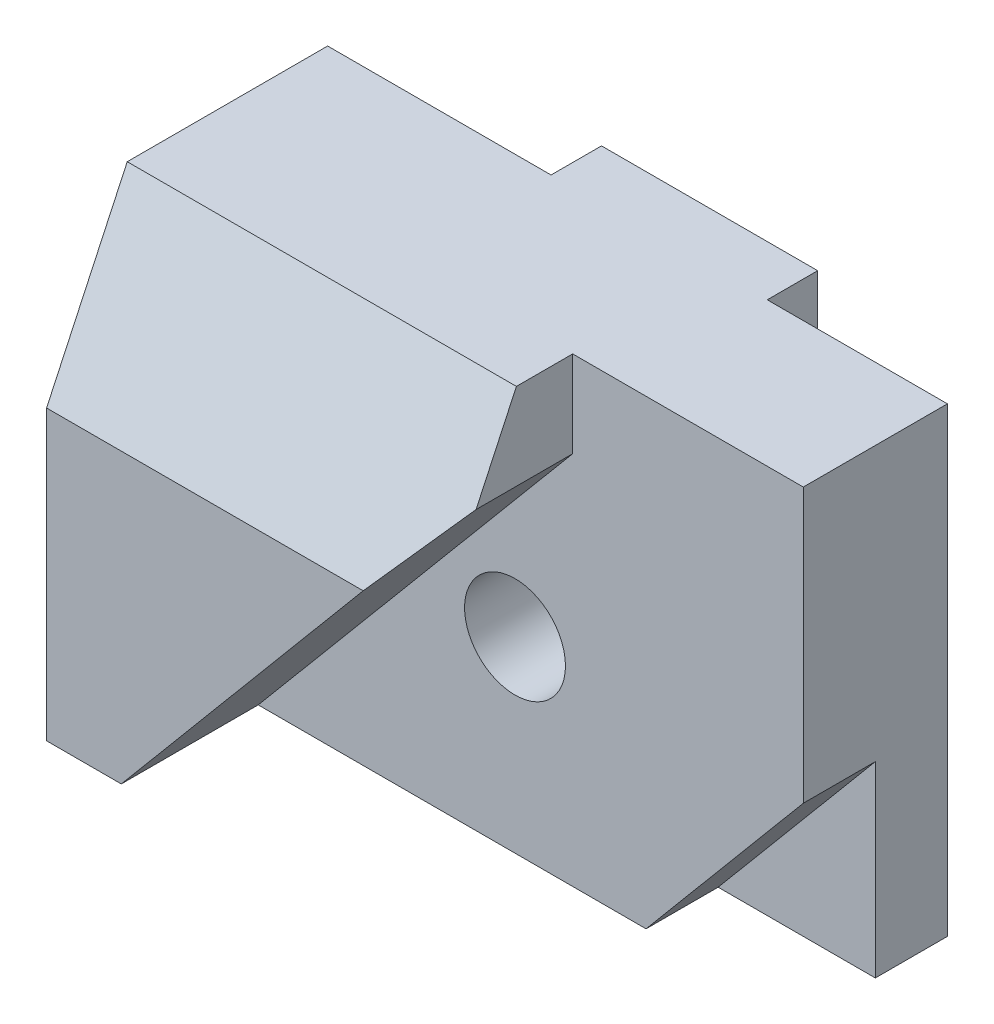
ISO-10303-21;
HEADER;
FILE_DESCRIPTION(('STEP AP214'),'2;1');
FILE_NAME('part.step','',(''),(''),'','','');
FILE_SCHEMA(('AUTOMOTIVE_DESIGN { 1 0 10303 214 1 1 1 1 }'));
ENDSEC;
DATA;
#1=APPLICATION_CONTEXT('core data for automotive mechanical design processes');
#2=APPLICATION_PROTOCOL_DEFINITION('international standard','automotive_design',2000,#1);
#3=PRODUCT_CONTEXT('',#1,'mechanical');
#4=PRODUCT('Part','Part','',(#3));
#5=PRODUCT_RELATED_PRODUCT_CATEGORY('part','',(#4));
#6=PRODUCT_DEFINITION_FORMATION('','',#4);
#7=PRODUCT_DEFINITION_CONTEXT('part definition',#1,'design');
#8=PRODUCT_DEFINITION('design','',#6,#7);
#9=PRODUCT_DEFINITION_SHAPE('','',#8);
#10=(LENGTH_UNIT() NAMED_UNIT(*) SI_UNIT(.MILLI.,.METRE.));
#11=(NAMED_UNIT(*) PLANE_ANGLE_UNIT() SI_UNIT($,.RADIAN.));
#12=(NAMED_UNIT(*) SI_UNIT($,.STERADIAN.) SOLID_ANGLE_UNIT());
#13=UNCERTAINTY_MEASURE_WITH_UNIT(LENGTH_MEASURE(1.E-05),#10,'distance_accuracy_value','');
#14=(GEOMETRIC_REPRESENTATION_CONTEXT(3) GLOBAL_UNCERTAINTY_ASSIGNED_CONTEXT((#13)) GLOBAL_UNIT_ASSIGNED_CONTEXT((#10,
#11,#12)) REPRESENTATION_CONTEXT('',''));
#15=CARTESIAN_POINT('',(0.,0.,0.));
#16=DIRECTION('',(0.,0.,1.));
#17=DIRECTION('',(1.,0.,0.));
#18=AXIS2_PLACEMENT_3D('',#15,#16,#17);
#19=CARTESIAN_POINT('',(0.,0.,0.));
#20=DIRECTION('',(0.,0.,-1.));
#21=DIRECTION('',(-1.,0.,0.));
#22=AXIS2_PLACEMENT_3D('',#19,#20,#21);
#23=PLANE('',#22);
#24=DIRECTION('',(-1.,0.,0.));
#25=VECTOR('',#24,1.);
#26=CARTESIAN_POINT('',(0.,64.,0.));
#27=LINE('',#26,#25);
#28=CARTESIAN_POINT('',(31.,64.,0.));
#29=VERTEX_POINT('',#28);
#30=CARTESIAN_POINT('',(0.,64.,0.));
#31=VERTEX_POINT('',#30);
#32=EDGE_CURVE('E178',#29,#31,#27,.T.);
#33=ORIENTED_EDGE('',*,*,#32,.F.);
#34=DIRECTION('',(0.,-1.,0.));
#35=VECTOR('',#34,1.);
#36=CARTESIAN_POINT('',(31.,64.,0.));
#37=LINE('',#36,#35);
#38=CARTESIAN_POINT('',(31.,0.,0.));
#39=VERTEX_POINT('',#38);
#40=EDGE_CURVE('E166',#29,#39,#37,.T.);
#41=ORIENTED_EDGE('',*,*,#40,.T.);
#42=DIRECTION('',(1.,0.,0.));
#43=VECTOR('',#42,1.);
#44=CARTESIAN_POINT('',(86.,0.,0.));
#45=LINE('',#44,#43);
#46=CARTESIAN_POINT('',(0.,0.,0.));
#47=VERTEX_POINT('',#46);
#48=EDGE_CURVE('E203',#47,#39,#45,.T.);
#49=ORIENTED_EDGE('',*,*,#48,.F.);
#50=DIRECTION('',(0.,-1.,0.));
#51=VECTOR('',#50,1.);
#52=CARTESIAN_POINT('',(0.,0.,0.));
#53=LINE('',#52,#51);
#54=EDGE_CURVE('E179',#31,#47,#53,.T.);
#55=ORIENTED_EDGE('',*,*,#54,.F.);
#56=EDGE_LOOP('',(#33,#41,#49,#55));
#57=FACE_BOUND('',#56,.T.);
#58=ADVANCED_FACE('F50',(#57),#23,.T.);
#59=CARTESIAN_POINT('',(0.,0.,20.));
#60=DIRECTION('',(0.,0.,1.));
#61=DIRECTION('',(1.,0.,0.));
#62=AXIS2_PLACEMENT_3D('',#59,#60,#61);
#63=PLANE('',#62);
#64=DIRECTION('',(-0.64278760968654,-0.766044443118977,0.));
#65=VECTOR('',#64,1.);
#66=CARTESIAN_POINT('',(86.,26.,20.));
#67=LINE('',#66,#65);
#68=CARTESIAN_POINT('',(86.,26.,20.));
#69=VERTEX_POINT('',#68);
#70=CARTESIAN_POINT('',(64.1834095893907,0.,20.));
#71=VERTEX_POINT('',#70);
#72=EDGE_CURVE('E248',#69,#71,#67,.T.);
#73=ORIENTED_EDGE('',*,*,#72,.F.);
#74=DIRECTION('',(0.,1.,0.));
#75=VECTOR('',#74,1.);
#76=CARTESIAN_POINT('',(86.,0.,20.));
#77=LINE('',#76,#75);
#78=CARTESIAN_POINT('',(86.,64.,20.));
#79=VERTEX_POINT('',#78);
#80=EDGE_CURVE('E204',#69,#79,#77,.T.);
#81=ORIENTED_EDGE('',*,*,#80,.T.);
#82=DIRECTION('',(-1.,0.,0.));
#83=VECTOR('',#82,1.);
#84=CARTESIAN_POINT('',(86.,64.,20.));
#85=LINE('',#84,#83);
#86=CARTESIAN_POINT('',(54.,64.,20.));
#87=VERTEX_POINT('',#86);
#88=EDGE_CURVE('E209',#79,#87,#85,.T.);
#89=ORIENTED_EDGE('',*,*,#88,.T.);
#90=DIRECTION('',(0.,-1.,0.));
#91=VECTOR('',#90,1.);
#92=CARTESIAN_POINT('',(54.,0.,20.));
#93=LINE('',#92,#91);
#94=CARTESIAN_POINT('',(54.,52.,20.));
#95=VERTEX_POINT('',#94);
#96=EDGE_CURVE('E219',#87,#95,#93,.T.);
#97=ORIENTED_EDGE('',*,*,#96,.T.);
#98=DIRECTION('',(-0.64278760968654,-0.766044443118977,0.));
#99=VECTOR('',#98,1.);
#100=CARTESIAN_POINT('',(6.08349921868961,-5.10466195066974,20.));
#101=LINE('',#100,#99);
#102=CARTESIAN_POINT('',(10.3668191787813,0.,20.));
#103=VERTEX_POINT('',#102);
#104=EDGE_CURVE('E221',#95,#103,#101,.T.);
#105=ORIENTED_EDGE('',*,*,#104,.T.);
#106=DIRECTION('',(1.,0.,0.));
#107=VECTOR('',#106,1.);
#108=CARTESIAN_POINT('',(0.,0.,20.));
#109=LINE('',#108,#107);
#110=EDGE_CURVE('E210',#103,#71,#109,.T.);
#111=ORIENTED_EDGE('',*,*,#110,.T.);
#112=EDGE_LOOP('',(#73,#81,#89,#97,#105,#111));
#113=FACE_BOUND('',#112,.T.);
#114=CARTESIAN_POINT('',(46.,26.,20.));
#115=DIRECTION('',(0.,0.,1.));
#116=DIRECTION('',(1.,0.,0.));
#117=AXIS2_PLACEMENT_3D('',#114,#115,#116);
#118=CIRCLE('',#117,7.);
#119=CARTESIAN_POINT('',(53.,26.,20.));
#120=VERTEX_POINT('',#119);
#121=EDGE_CURVE('E238',#120,#120,#118,.T.);
#122=ORIENTED_EDGE('',*,*,#121,.F.);
#123=EDGE_LOOP('',(#122));
#124=FACE_BOUND('',#123,.T.);
#125=ADVANCED_FACE('F275',(#113,#124),#63,.T.);
#126=CARTESIAN_POINT('',(86.,0.,10.));
#127=DIRECTION('',(0.,1.,0.));
#128=DIRECTION('',(0.,0.,1.));
#129=AXIS2_PLACEMENT_3D('',#126,#127,#128);
#130=PLANE('',#129);
#131=DIRECTION('',(1.,0.,0.));
#132=VECTOR('',#131,1.);
#133=CARTESIAN_POINT('',(86.,0.,10.));
#134=LINE('',#133,#132);
#135=CARTESIAN_POINT('',(64.1834095893907,0.,10.));
#136=VERTEX_POINT('',#135);
#137=CARTESIAN_POINT('',(86.,0.,10.));
#138=VERTEX_POINT('',#137);
#139=EDGE_CURVE('E72',#136,#138,#134,.T.);
#140=ORIENTED_EDGE('',*,*,#139,.F.);
#141=DIRECTION('',(0.,0.,1.));
#142=VECTOR('',#141,1.);
#143=CARTESIAN_POINT('',(64.1834095893907,0.,10.));
#144=LINE('',#143,#142);
#145=EDGE_CURVE('E241',#136,#71,#144,.T.);
#146=ORIENTED_EDGE('',*,*,#145,.T.);
#147=ORIENTED_EDGE('',*,*,#110,.F.);
#148=DIRECTION('',(0.,0.,-1.));
#149=VECTOR('',#148,1.);
#150=CARTESIAN_POINT('',(10.3668191787813,0.,39.));
#151=LINE('',#150,#149);
#152=CARTESIAN_POINT('',(10.3668191787813,0.,39.));
#153=VERTEX_POINT('',#152);
#154=EDGE_CURVE('E220',#153,#103,#151,.T.);
#155=ORIENTED_EDGE('',*,*,#154,.F.);
#156=DIRECTION('',(1.,0.,0.));
#157=VECTOR('',#156,1.);
#158=CARTESIAN_POINT('',(0.,0.,39.));
#159=LINE('',#158,#157);
#160=CARTESIAN_POINT('',(0.,0.,39.));
#161=VERTEX_POINT('',#160);
#162=EDGE_CURVE('E218',#161,#153,#159,.T.);
#163=ORIENTED_EDGE('',*,*,#162,.F.);
#164=DIRECTION('',(0.,0.,-1.));
#165=VECTOR('',#164,1.);
#166=CARTESIAN_POINT('',(0.,0.,10.));
#167=LINE('',#166,#165);
#168=EDGE_CURVE('E182',#161,#47,#167,.T.);
#169=ORIENTED_EDGE('',*,*,#168,.T.);
#170=ORIENTED_EDGE('',*,*,#48,.T.);
#171=DIRECTION('',(0.,0.,-1.));
#172=VECTOR('',#171,1.);
#173=CARTESIAN_POINT('',(31.,0.,0.));
#174=LINE('',#173,#172);
#175=CARTESIAN_POINT('',(31.,0.,-7.));
#176=VERTEX_POINT('',#175);
#177=EDGE_CURVE('E61',#39,#176,#174,.T.);
#178=ORIENTED_EDGE('',*,*,#177,.T.);
#179=DIRECTION('',(1.,0.,0.));
#180=VECTOR('',#179,1.);
#181=CARTESIAN_POINT('',(31.,0.,-7.));
#182=LINE('',#181,#180);
#183=CARTESIAN_POINT('',(61.,0.,-7.));
#184=VERTEX_POINT('',#183);
#185=EDGE_CURVE('E159',#176,#184,#182,.T.);
#186=ORIENTED_EDGE('',*,*,#185,.T.);
#187=DIRECTION('',(0.,0.,1.));
#188=VECTOR('',#187,1.);
#189=CARTESIAN_POINT('',(61.,0.,0.));
#190=LINE('',#189,#188);
#191=CARTESIAN_POINT('',(61.,0.,0.));
#192=VERTEX_POINT('',#191);
#193=EDGE_CURVE('E261',#184,#192,#190,.T.);
#194=ORIENTED_EDGE('',*,*,#193,.T.);
#195=CARTESIAN_POINT('',(86.,0.,0.));
#196=VERTEX_POINT('',#195);
#197=EDGE_CURVE('E169',#192,#196,#45,.T.);
#198=ORIENTED_EDGE('',*,*,#197,.T.);
#199=DIRECTION('',(0.,0.,-1.));
#200=VECTOR('',#199,1.);
#201=CARTESIAN_POINT('',(86.,0.,10.));
#202=LINE('',#201,#200);
#203=EDGE_CURVE('E57',#138,#196,#202,.T.);
#204=ORIENTED_EDGE('',*,*,#203,.F.);
#205=EDGE_LOOP('',(#140,#146,#147,#155,#163,#169,#170,#178,#186,#194,#198,#204));
#206=FACE_BOUND('',#205,.T.);
#207=ADVANCED_FACE('F47',(#206),#130,.F.);
#208=CARTESIAN_POINT('',(86.,64.,10.));
#209=DIRECTION('',(-1.,0.,0.));
#210=DIRECTION('',(0.,0.,1.));
#211=AXIS2_PLACEMENT_3D('',#208,#209,#210);
#212=PLANE('',#211);
#213=ORIENTED_EDGE('',*,*,#80,.F.);
#214=DIRECTION('',(0.,0.,1.));
#215=VECTOR('',#214,1.);
#216=CARTESIAN_POINT('',(86.,26.,10.));
#217=LINE('',#216,#215);
#218=CARTESIAN_POINT('',(86.,26.,10.));
#219=VERTEX_POINT('',#218);
#220=EDGE_CURVE('E242',#219,#69,#217,.T.);
#221=ORIENTED_EDGE('',*,*,#220,.F.);
#222=DIRECTION('',(0.,1.,0.));
#223=VECTOR('',#222,1.);
#224=CARTESIAN_POINT('',(86.,0.,10.));
#225=LINE('',#224,#223);
#226=EDGE_CURVE('E200',#138,#219,#225,.T.);
#227=ORIENTED_EDGE('',*,*,#226,.F.);
#228=ORIENTED_EDGE('',*,*,#203,.T.);
#229=DIRECTION('',(0.,1.,0.));
#230=VECTOR('',#229,1.);
#231=CARTESIAN_POINT('',(86.,64.,0.));
#232=LINE('',#231,#230);
#233=CARTESIAN_POINT('',(86.,64.,0.));
#234=VERTEX_POINT('',#233);
#235=EDGE_CURVE('E181',#196,#234,#232,.T.);
#236=ORIENTED_EDGE('',*,*,#235,.T.);
#237=DIRECTION('',(0.,0.,-1.));
#238=VECTOR('',#237,1.);
#239=CARTESIAN_POINT('',(86.,64.,10.));
#240=LINE('',#239,#238);
#241=EDGE_CURVE('E177',#79,#234,#240,.T.);
#242=ORIENTED_EDGE('',*,*,#241,.F.);
#243=EDGE_LOOP('',(#213,#221,#227,#228,#236,#242));
#244=FACE_BOUND('',#243,.T.);
#245=ADVANCED_FACE('F197',(#244),#212,.F.);
#246=CARTESIAN_POINT('',(0.,64.,10.));
#247=DIRECTION('',(0.,-1.,0.));
#248=DIRECTION('',(0.,0.,-1.));
#249=AXIS2_PLACEMENT_3D('',#246,#247,#248);
#250=PLANE('',#249);
#251=DIRECTION('',(0.,0.,-1.));
#252=VECTOR('',#251,1.);
#253=CARTESIAN_POINT('',(0.,64.,10.));
#254=LINE('',#253,#252);
#255=CARTESIAN_POINT('',(0.,64.,27.8086162042802));
#256=VERTEX_POINT('',#255);
#257=EDGE_CURVE('E187',#256,#31,#254,.T.);
#258=ORIENTED_EDGE('',*,*,#257,.F.);
#259=DIRECTION('',(-1.,0.,0.));
#260=VECTOR('',#259,1.);
#261=CARTESIAN_POINT('',(65.,64.,27.8086162042802));
#262=LINE('',#261,#260);
#263=CARTESIAN_POINT('',(54.,64.,27.8086162042802));
#264=VERTEX_POINT('',#263);
#265=EDGE_CURVE('E237',#264,#256,#262,.T.);
#266=ORIENTED_EDGE('',*,*,#265,.F.);
#267=DIRECTION('',(0.,0.,-1.));
#268=VECTOR('',#267,1.);
#269=CARTESIAN_POINT('',(54.,64.,39.));
#270=LINE('',#269,#268);
#271=EDGE_CURVE('E214',#264,#87,#270,.T.);
#272=ORIENTED_EDGE('',*,*,#271,.T.);
#273=ORIENTED_EDGE('',*,*,#88,.F.);
#274=ORIENTED_EDGE('',*,*,#241,.T.);
#275=CARTESIAN_POINT('',(61.,64.,0.));
#276=VERTEX_POINT('',#275);
#277=EDGE_CURVE('E170',#234,#276,#27,.T.);
#278=ORIENTED_EDGE('',*,*,#277,.T.);
#279=DIRECTION('',(0.,0.,1.));
#280=VECTOR('',#279,1.);
#281=CARTESIAN_POINT('',(61.,64.,0.));
#282=LINE('',#281,#280);
#283=CARTESIAN_POINT('',(61.,64.,-7.));
#284=VERTEX_POINT('',#283);
#285=EDGE_CURVE('E146',#284,#276,#282,.T.);
#286=ORIENTED_EDGE('',*,*,#285,.F.);
#287=DIRECTION('',(1.,0.,0.));
#288=VECTOR('',#287,1.);
#289=CARTESIAN_POINT('',(31.,64.,-7.));
#290=LINE('',#289,#288);
#291=CARTESIAN_POINT('',(31.,64.,-7.));
#292=VERTEX_POINT('',#291);
#293=EDGE_CURVE('E168',#292,#284,#290,.T.);
#294=ORIENTED_EDGE('',*,*,#293,.F.);
#295=DIRECTION('',(0.,0.,-1.));
#296=VECTOR('',#295,1.);
#297=CARTESIAN_POINT('',(31.,64.,0.));
#298=LINE('',#297,#296);
#299=EDGE_CURVE('E157',#29,#292,#298,.T.);
#300=ORIENTED_EDGE('',*,*,#299,.F.);
#301=ORIENTED_EDGE('',*,*,#32,.T.);
#302=EDGE_LOOP('',(#258,#266,#272,#273,#274,#278,#286,#294,#300,#301));
#303=FACE_BOUND('',#302,.T.);
#304=ADVANCED_FACE('F172',(#303),#250,.F.);
#305=CARTESIAN_POINT('',(0.,0.,10.));
#306=DIRECTION('',(1.,0.,0.));
#307=DIRECTION('',(0.,0.,-1.));
#308=AXIS2_PLACEMENT_3D('',#305,#306,#307);
#309=PLANE('',#308);
#310=DIRECTION('',(0.,-1.,0.));
#311=VECTOR('',#310,1.);
#312=CARTESIAN_POINT('',(0.,0.,39.));
#313=LINE('',#312,#311);
#314=CARTESIAN_POINT('',(0.,40.,39.));
#315=VERTEX_POINT('',#314);
#316=EDGE_CURVE('E229',#315,#161,#313,.T.);
#317=ORIENTED_EDGE('',*,*,#316,.F.);
#318=DIRECTION('',(0.,-0.906307787036653,0.422618261740694));
#319=VECTOR('',#318,1.);
#320=CARTESIAN_POINT('',(0.,40.,39.));
#321=LINE('',#320,#319);
#322=EDGE_CURVE('E236',#256,#315,#321,.T.);
#323=ORIENTED_EDGE('',*,*,#322,.F.);
#324=ORIENTED_EDGE('',*,*,#257,.T.);
#325=ORIENTED_EDGE('',*,*,#54,.T.);
#326=ORIENTED_EDGE('',*,*,#168,.F.);
#327=EDGE_LOOP('',(#317,#323,#324,#325,#326));
#328=FACE_BOUND('',#327,.T.);
#329=ADVANCED_FACE('F288',(#328),#309,.F.);
#330=DIRECTION('',(0.,-1.,0.));
#331=VECTOR('',#330,1.);
#332=CARTESIAN_POINT('',(61.,64.,0.));
#333=LINE('',#332,#331);
#334=EDGE_CURVE('E155',#276,#192,#333,.T.);
#335=ORIENTED_EDGE('',*,*,#334,.F.);
#336=ORIENTED_EDGE('',*,*,#277,.F.);
#337=ORIENTED_EDGE('',*,*,#235,.F.);
#338=ORIENTED_EDGE('',*,*,#197,.F.);
#339=EDGE_LOOP('',(#335,#336,#337,#338));
#340=FACE_BOUND('',#339,.T.);
#341=ADVANCED_FACE('F164',(#340),#23,.T.);
#342=CARTESIAN_POINT('',(6.08349921868961,-5.10466195066974,39.));
#343=DIRECTION('',(0.766044443118977,-0.64278760968654,0.));
#344=DIRECTION('',(0.64278760968654,0.766044443118977,0.));
#345=AXIS2_PLACEMENT_3D('',#342,#343,#344);
#346=PLANE('',#345);
#347=DIRECTION('',(0.605326699380344,0.721400268679718,-0.336394469880421));
#348=VECTOR('',#347,1.);
#349=CARTESIAN_POINT('',(10.3663471826026,-0.000562503141664575,57.6525686257223));
#350=LINE('',#349,#348);
#351=CARTESIAN_POINT('',(43.9308044258726,40.,39.));
#352=VERTEX_POINT('',#351);
#353=CARTESIAN_POINT('',(54.,52.,33.4043081021401));
#354=VERTEX_POINT('',#353);
#355=EDGE_CURVE('E230',#352,#354,#350,.T.);
#356=ORIENTED_EDGE('',*,*,#355,.F.);
#357=DIRECTION('',(-0.64278760968654,-0.766044443118977,0.));
#358=VECTOR('',#357,1.);
#359=CARTESIAN_POINT('',(6.08349921868961,-5.10466195066974,39.));
#360=LINE('',#359,#358);
#361=EDGE_CURVE('E224',#352,#153,#360,.T.);
#362=ORIENTED_EDGE('',*,*,#361,.T.);
#363=ORIENTED_EDGE('',*,*,#154,.T.);
#364=ORIENTED_EDGE('',*,*,#104,.F.);
#365=DIRECTION('',(0.,0.,-1.));
#366=VECTOR('',#365,1.);
#367=CARTESIAN_POINT('',(54.,52.,39.));
#368=LINE('',#367,#366);
#369=EDGE_CURVE('E213',#354,#95,#368,.T.);
#370=ORIENTED_EDGE('',*,*,#369,.F.);
#371=EDGE_LOOP('',(#356,#362,#363,#364,#370));
#372=FACE_BOUND('',#371,.T.);
#373=ADVANCED_FACE('F289',(#372),#346,.T.);
#374=CARTESIAN_POINT('',(54.,0.,39.));
#375=DIRECTION('',(1.,0.,0.));
#376=DIRECTION('',(0.,0.,-1.));
#377=AXIS2_PLACEMENT_3D('',#374,#375,#376);
#378=PLANE('',#377);
#379=DIRECTION('',(0.,0.906307787036653,-0.422618261740694));
#380=VECTOR('',#379,1.);
#381=CARTESIAN_POINT('',(54.,7.14424780626902,54.3208888623794));
#382=LINE('',#381,#380);
#383=EDGE_CURVE('E233',#354,#264,#382,.T.);
#384=ORIENTED_EDGE('',*,*,#383,.F.);
#385=ORIENTED_EDGE('',*,*,#369,.T.);
#386=ORIENTED_EDGE('',*,*,#96,.F.);
#387=ORIENTED_EDGE('',*,*,#271,.F.);
#388=EDGE_LOOP('',(#384,#385,#386,#387));
#389=FACE_BOUND('',#388,.T.);
#390=ADVANCED_FACE('F294',(#389),#378,.T.);
#391=CARTESIAN_POINT('',(0.,0.,39.));
#392=DIRECTION('',(0.,0.,1.));
#393=DIRECTION('',(1.,0.,0.));
#394=AXIS2_PLACEMENT_3D('',#391,#392,#393);
#395=PLANE('',#394);
#396=DIRECTION('',(1.,0.,0.));
#397=VECTOR('',#396,1.);
#398=CARTESIAN_POINT('',(0.,40.,39.));
#399=LINE('',#398,#397);
#400=EDGE_CURVE('E11',#315,#352,#399,.T.);
#401=ORIENTED_EDGE('',*,*,#400,.F.);
#402=ORIENTED_EDGE('',*,*,#316,.T.);
#403=ORIENTED_EDGE('',*,*,#162,.T.);
#404=ORIENTED_EDGE('',*,*,#361,.F.);
#405=EDGE_LOOP('',(#401,#402,#403,#404));
#406=FACE_BOUND('',#405,.T.);
#407=ADVANCED_FACE('F306',(#406),#395,.T.);
#408=CARTESIAN_POINT('',(65.,40.,39.));
#409=DIRECTION('',(0.,-0.422618261740694,-0.906307787036653));
#410=DIRECTION('',(0.,0.906307787036653,-0.422618261740694));
#411=AXIS2_PLACEMENT_3D('',#408,#409,#410);
#412=PLANE('',#411);
#413=ORIENTED_EDGE('',*,*,#355,.T.);
#414=ORIENTED_EDGE('',*,*,#383,.T.);
#415=ORIENTED_EDGE('',*,*,#265,.T.);
#416=ORIENTED_EDGE('',*,*,#322,.T.);
#417=ORIENTED_EDGE('',*,*,#400,.T.);
#418=EDGE_LOOP('',(#413,#414,#415,#416,#417));
#419=FACE_BOUND('',#418,.T.);
#420=ADVANCED_FACE('F311',(#419),#412,.F.);
#421=CARTESIAN_POINT('',(46.,26.,-45.));
#422=DIRECTION('',(0.,0.,1.));
#423=DIRECTION('',(1.,0.,0.));
#424=AXIS2_PLACEMENT_3D('',#421,#422,#423);
#425=CYLINDRICAL_SURFACE('',#424,7.);
#426=ORIENTED_EDGE('',*,*,#121,.T.);
#427=EDGE_LOOP('',(#426));
#428=FACE_BOUND('',#427,.T.);
#429=CARTESIAN_POINT('',(46.,26.,-7.));
#430=DIRECTION('',(0.,0.,-1.));
#431=DIRECTION('',(-1.,0.,0.));
#432=AXIS2_PLACEMENT_3D('',#429,#430,#431);
#433=CIRCLE('',#432,7.);
#434=CARTESIAN_POINT('',(39.,26.,-7.));
#435=VERTEX_POINT('',#434);
#436=EDGE_CURVE('E51',#435,#435,#433,.T.);
#437=ORIENTED_EDGE('',*,*,#436,.T.);
#438=EDGE_LOOP('',(#437));
#439=FACE_BOUND('',#438,.T.);
#440=ADVANCED_FACE('F338',(#428,#439),#425,.F.);
#441=CARTESIAN_POINT('',(86.,26.,10.));
#442=DIRECTION('',(-0.766044443118977,0.64278760968654,0.));
#443=DIRECTION('',(-0.64278760968654,-0.766044443118977,0.));
#444=AXIS2_PLACEMENT_3D('',#441,#442,#443);
#445=PLANE('',#444);
#446=ORIENTED_EDGE('',*,*,#72,.T.);
#447=ORIENTED_EDGE('',*,*,#145,.F.);
#448=DIRECTION('',(-0.64278760968654,-0.766044443118977,0.));
#449=VECTOR('',#448,1.);
#450=CARTESIAN_POINT('',(86.,26.,10.));
#451=LINE('',#450,#449);
#452=EDGE_CURVE('E246',#219,#136,#451,.T.);
#453=ORIENTED_EDGE('',*,*,#452,.F.);
#454=ORIENTED_EDGE('',*,*,#220,.T.);
#455=EDGE_LOOP('',(#446,#447,#453,#454));
#456=FACE_BOUND('',#455,.T.);
#457=ADVANCED_FACE('F330',(#456),#445,.F.);
#458=CARTESIAN_POINT('',(0.,0.,10.));
#459=DIRECTION('',(0.,0.,-1.));
#460=DIRECTION('',(-1.,0.,0.));
#461=AXIS2_PLACEMENT_3D('',#458,#459,#460);
#462=PLANE('',#461);
#463=ORIENTED_EDGE('',*,*,#139,.T.);
#464=ORIENTED_EDGE('',*,*,#226,.T.);
#465=ORIENTED_EDGE('',*,*,#452,.T.);
#466=EDGE_LOOP('',(#463,#464,#465));
#467=FACE_BOUND('',#466,.T.);
#468=ADVANCED_FACE('F327',(#467),#462,.F.);
#469=CARTESIAN_POINT('',(31.,64.,0.));
#470=DIRECTION('',(-1.,0.,0.));
#471=DIRECTION('',(0.,0.,1.));
#472=AXIS2_PLACEMENT_3D('',#469,#470,#471);
#473=PLANE('',#472);
#474=ORIENTED_EDGE('',*,*,#177,.F.);
#475=ORIENTED_EDGE('',*,*,#40,.F.);
#476=ORIENTED_EDGE('',*,*,#299,.T.);
#477=DIRECTION('',(0.,-1.,0.));
#478=VECTOR('',#477,1.);
#479=CARTESIAN_POINT('',(31.,64.,-7.));
#480=LINE('',#479,#478);
#481=EDGE_CURVE('E254',#292,#176,#480,.T.);
#482=ORIENTED_EDGE('',*,*,#481,.T.);
#483=EDGE_LOOP('',(#474,#475,#476,#482));
#484=FACE_BOUND('',#483,.T.);
#485=ADVANCED_FACE('F266',(#484),#473,.T.);
#486=CARTESIAN_POINT('',(31.,64.,-7.));
#487=DIRECTION('',(0.,0.,-1.));
#488=DIRECTION('',(-1.,0.,0.));
#489=AXIS2_PLACEMENT_3D('',#486,#487,#488);
#490=PLANE('',#489);
#491=ORIENTED_EDGE('',*,*,#436,.F.);
#492=EDGE_LOOP('',(#491));
#493=FACE_BOUND('',#492,.T.);
#494=ORIENTED_EDGE('',*,*,#185,.F.);
#495=ORIENTED_EDGE('',*,*,#481,.F.);
#496=ORIENTED_EDGE('',*,*,#293,.T.);
#497=DIRECTION('',(0.,-1.,0.));
#498=VECTOR('',#497,1.);
#499=CARTESIAN_POINT('',(61.,64.,-7.));
#500=LINE('',#499,#498);
#501=EDGE_CURVE('E152',#284,#184,#500,.T.);
#502=ORIENTED_EDGE('',*,*,#501,.T.);
#503=EDGE_LOOP('',(#494,#495,#496,#502));
#504=FACE_BOUND('',#503,.T.);
#505=ADVANCED_FACE('F269',(#493,#504),#490,.T.);
#506=CARTESIAN_POINT('',(61.,64.,0.));
#507=DIRECTION('',(1.,0.,0.));
#508=DIRECTION('',(0.,0.,-1.));
#509=AXIS2_PLACEMENT_3D('',#506,#507,#508);
#510=PLANE('',#509);
#511=ORIENTED_EDGE('',*,*,#193,.F.);
#512=ORIENTED_EDGE('',*,*,#501,.F.);
#513=ORIENTED_EDGE('',*,*,#285,.T.);
#514=ORIENTED_EDGE('',*,*,#334,.T.);
#515=EDGE_LOOP('',(#511,#512,#513,#514));
#516=FACE_BOUND('',#515,.T.);
#517=ADVANCED_FACE('F151',(#516),#510,.T.);
#518=CLOSED_SHELL('',(#58,#125,#207,#245,#304,#329,#341,#373,#390,#407,#420,#440,#457,#468,#485,
#505,#517));
#519=MANIFOLD_SOLID_BREP('B2',#518);
#520=ADVANCED_BREP_SHAPE_REPRESENTATION('',(#18,#519),#14);
#521=SHAPE_DEFINITION_REPRESENTATION(#9,#520);
ENDSEC;
END-ISO-10303-21;
